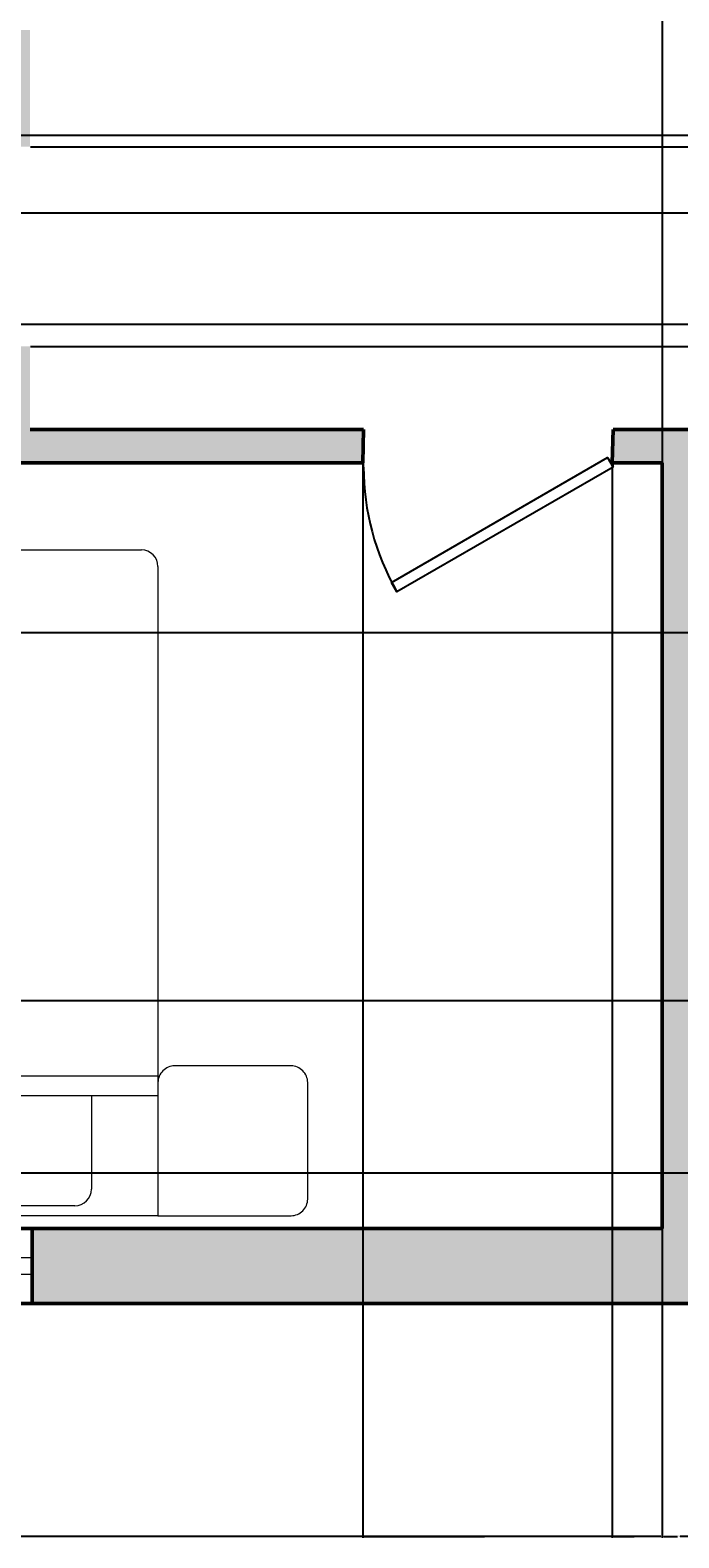
# Model space of a CAD drawing. Units: inches. Extents: x 1869 to 2483, y 2084 to 2479.
# Tile 2 of 7: x 2010 to 2088, y 2084 to 2265. Entities that reach past the tile are written whole.
import ezdxf

# ---------------------------------------------------------------- set-up
doc = ezdxf.new("R2010")
doc.units = ezdxf.units.IN
for name, color, linetype, lineweight in [('A-ANNO-DIMS', 2, 'Continuous', 18), ('A-DOOR', 3, 'Continuous', 25), ('A-FURN', 8, 'Continuous', 18), ('A-GLAZ', 4, 'Continuous', 18), ('A-WALL', 7, 'Continuous', 50)]:
    doc.layers.add(name, color=color, linetype=linetype, lineweight=lineweight)
doc.layers.add('A-WALL-PATT', color=18, linetype='Continuous', lineweight=13, true_color=0x000000)
doc.styles.get("Standard").update_dxf_attribs({"font": 'arial.ttf'})
doc.dimstyles.get("Standard").update_dxf_attribs({"dimtxt": 0.18, "dimasz": 0.18, "dimexe": 0.18, "dimexo": 0.0625, "dimgap": 0.09, "dimtad": 0, "dimtih": 1, "dimtoh": 1, "dimdec": 4, "dimzin": 0, "dimdsep": 46, "dimtxsty": 'Standard', "dimcen": 0.09, "dimadec": 0, "dimazin": 0, "dimtfac": 1, "dimtdec": 4, "dimtofl": 0, "dimtmove": 0, "dimatfit": 3, "dimfxl": 1, "dimtolj": 1, "dimtzin": 0, "dimarcsym": 0})

# ---------------------------------------------------------------- blocks, each defined once
blk = doc.blocks.new('Bed - Queen')
for p, q in [((0, -78), (0, 0)), ((0, 0), (60, 0)), ((60, 0), (60, -78)), ((10, -1.2), (26.8, -1.2)), ((33.2, -1.2), (50, -1.2)), ((8, -14.4), (8, -3.2)), ((28.8, -3.2), (28.8, -14.4)), ((31.2, -14.4), (31.2, -3.2)), ((52, -3.2), (52, -14.4)), ((0, -14.4), (44.8, -14.4)), ((60, -29.6), (44.8, -14.4)), ((44.8, -14.4), (44.8, -27.6)), ((44.8, -16.8), (0, -16.8)), ((50, -16.4), (46.8, -16.4)), ((46.8, -29.6), (60, -29.6)), ((58, -80), (2, -80))]:
    blk.add_line(p, q)
for points in [[(0, 0), (-16, 0, 0.414214), (-18, -2), (-18, -16, 0.414214), (-16, -18), (-2, -18, 0.414214), (0, -16)], [(75.96, 0.02), (59.96, 0.02), (59.96, -15.98, 0.414214), (61.96, -17.98), (75.96, -17.98, 0.414214), (77.96, -15.98), (77.96, -1.98, 0.414214)]]:
    blk.add_lwpolyline(points, format="xyb", close=True)
for centre, start, end in [((10, -3.2), 90, 180), ((26.8, -3.2), 0, 90), ((33.2, -3.2), 90, 180), ((50, -3.2), 0, 90), ((50, -14.4), 270, 0), ((46.8, -27.6), 180, 270), ((2, -78), 180, 270), ((58, -78), 270, 0)]:
    blk.add_arc(centre, 2, start, end)
blk = doc.blocks.new('*U14')
for p, q in [((-40, 0), (-40, 6)), ((0, 0), (0, 6))]:
    blk.add_line(p, q)
blk.add_lwpolyline([(0, 0), (-34.64, -20), (-35.52, -18.48), (-0.88, 1.52)], close=True)
blk.add_arc((0, 0), 40, 180, 210)
blk = doc.blocks.new('WIN-GLAZING-48IN')
for p, q in [((0, 2), (48, 2)), ((0, 0), (48, 0))]:
    blk.add_line(p, q)
blk = doc.blocks.new('*D40')
at = {"layer": 'A-ANNO-DIMS', "color": 0, "lineweight": -2, "transparency": 16777216}
for p, q in [((1906.08, 2120.66), (1906.08, 2083.54)), ((2086.08, 2120.66), (2086.08, 2083.54)), ((1906.26, 2083.72), (1995.8, 2083.72)), ((2085.9, 2083.72), (1996.36, 2083.72))]:
    blk.add_line(p, q, dxfattribs=at)
at = {"layer": 'A-ANNO-DIMS', "color": 0, "transparency": 16777216}
for points in [[(1906.26, 2083.75), (1906.26, 2083.69), (1906.08, 2083.72)], [(2085.9, 2083.75), (2085.9, 2083.69), (2086.08, 2083.72)]]:
    blk.add_solid(points, dxfattribs=at)
at = {"layer": 'Defpoints', "color": 0, "transparency": 16777216}
for p in [(1906.08, 2120.72), (2086.08, 2120.72), (2086.08, 2083.72)]:
    blk.add_point(p, dxfattribs=at)
at = {"layer": 'A-ANNO-DIMS', "color": 0, "transparency": 16777216, "insert": (1996.08, 2083.72), "char_height": 0.18, "attachment_point": 5}
blk.add_mtext('\\A1;180', dxfattribs=at)
blk = doc.blocks.new('*D57')
at = {"layer": 'A-ANNO-DIMS', "color": 0, "lineweight": -2, "transparency": 16777216}
for p, q in [((2446.02, 2296.72), (1868.9, 2296.72)), ((1869.08, 2296.54), (1869.08, 2274.58)), ((1869.08, 2252.25), (1869.08, 2274.22)), ((2446.02, 2252.07), (1868.9, 2252.07))]:
    blk.add_line(p, q, dxfattribs=at)
at = {"layer": 'A-ANNO-DIMS', "color": 0, "transparency": 16777216}
for points in [[(1869.05, 2296.54), (1869.11, 2296.54), (1869.08, 2296.72)], [(1869.05, 2252.25), (1869.11, 2252.25), (1869.08, 2252.07)]]:
    blk.add_solid(points, dxfattribs=at)
at = {"layer": 'Defpoints', "color": 0, "transparency": 16777216}
for p in [(1869.08, 2296.72), (2446.08, 2296.72), (2446.08, 2252.07)]:
    blk.add_point(p, dxfattribs=at)
at = {"layer": 'A-ANNO-DIMS', "color": 0, "transparency": 16777216, "insert": (1869.08, 2274.4), "char_height": 0.18, "attachment_point": 5}
blk.add_mtext('\\A1;44.65', dxfattribs=at)
blk = doc.blocks.new('*D63')
at = {"layer": 'A-ANNO-DIMS', "color": 0, "lineweight": -2, "transparency": 16777216}
for p, q in [((2348.34, 2272.72), (1868.9, 2272.72)), ((1869.08, 2272.54), (1869.08, 2257.91)), ((1869.08, 2242.9), (1869.08, 2257.54)), ((2348.34, 2242.72), (1868.9, 2242.72))]:
    blk.add_line(p, q, dxfattribs=at)
at = {"layer": 'A-ANNO-DIMS', "color": 0, "transparency": 16777216}
for points in [[(1869.05, 2272.54), (1869.11, 2272.54), (1869.08, 2272.72)], [(1869.05, 2242.9), (1869.11, 2242.9), (1869.08, 2242.72)]]:
    blk.add_solid(points, dxfattribs=at)
at = {"layer": 'Defpoints', "color": 0, "transparency": 16777216}
for p in [(1869.08, 2272.72), (2348.4, 2272.72), (2348.4, 2242.72)]:
    blk.add_point(p, dxfattribs=at)
at = {"layer": 'A-ANNO-DIMS', "color": 0, "transparency": 16777216, "insert": (1869.08, 2257.72), "char_height": 0.18, "attachment_point": 5}
blk.add_mtext('\\A1;30', dxfattribs=at)
blk = doc.blocks.new('*D66')
at = {"layer": 'A-ANNO-DIMS', "color": 0, "lineweight": -2, "transparency": 16777216}
for p, q in [((2050.07, 2212.66), (2050.07, 2083.54)), ((2080.08, 2212.66), (2080.08, 2083.54)), ((2050.25, 2083.72), (2064.7, 2083.72)), ((2079.9, 2083.72), (2065.45, 2083.72))]:
    blk.add_line(p, q, dxfattribs=at)
at = {"layer": 'A-ANNO-DIMS', "color": 0, "transparency": 16777216}
for points in [[(2050.25, 2083.75), (2050.25, 2083.69), (2050.07, 2083.72)], [(2079.9, 2083.75), (2079.9, 2083.69), (2080.08, 2083.72)]]:
    blk.add_solid(points, dxfattribs=at)
at = {"layer": 'Defpoints', "color": 0, "transparency": 16777216}
for p in [(2050.07, 2212.72), (2080.08, 2212.72), (2080.08, 2083.72)]:
    blk.add_point(p, dxfattribs=at)
at = {"layer": 'A-ANNO-DIMS', "color": 0, "transparency": 16777216, "insert": (2065.07, 2083.72), "char_height": 0.18, "attachment_point": 5}
blk.add_mtext('\\A1;30.01', dxfattribs=at)
blk = doc.blocks.new('*D68')
at = {"layer": 'A-ANNO-DIMS', "color": 0, "lineweight": -2, "transparency": 16777216}
for p, q in [((2010.14, 2250.72), (2483.26, 2250.72)), ((2483.08, 2250.54), (2483.08, 2238.9)), ((2483.08, 2226.9), (2483.08, 2238.54)), ((2010.14, 2226.72), (2483.26, 2226.72))]:
    blk.add_line(p, q, dxfattribs=at)
at = {"layer": 'A-ANNO-DIMS', "color": 0, "transparency": 16777216}
for points in [[(2483.05, 2250.54), (2483.11, 2250.54), (2483.08, 2250.72)], [(2483.05, 2226.9), (2483.11, 2226.9), (2483.08, 2226.72)]]:
    blk.add_solid(points, dxfattribs=at)
at = {"layer": 'Defpoints', "color": 0, "transparency": 16777216}
for p in [(2010.08, 2250.72), (2483.08, 2250.72), (2010.08, 2226.72)]:
    blk.add_point(p, dxfattribs=at)
at = {"layer": 'A-ANNO-DIMS', "color": 0, "transparency": 16777216, "insert": (2483.08, 2238.72), "char_height": 0.18, "attachment_point": 5}
blk.add_mtext('\\A1;24', dxfattribs=at)
blk = doc.blocks.new('*D72')
at = {"layer": 'A-ANNO-DIMS', "color": 0, "lineweight": -2, "transparency": 16777216}
for p, q in [((2086.08, 2300.66), (2086.08, 2083.54)), ((2090.08, 2296.66), (2090.08, 2083.54)), ((2086.26, 2083.72), (2087.93, 2083.72)), ((2089.9, 2083.72), (2088.23, 2083.72))]:
    blk.add_line(p, q, dxfattribs=at)
at = {"layer": 'A-ANNO-DIMS', "color": 0, "transparency": 16777216}
for points in [[(2086.26, 2083.75), (2086.26, 2083.69), (2086.08, 2083.72)], [(2089.9, 2083.75), (2089.9, 2083.69), (2090.08, 2083.72)]]:
    blk.add_solid(points, dxfattribs=at)
at = {"layer": 'Defpoints', "color": 0, "transparency": 16777216}
for p in [(2086.08, 2300.72), (2090.08, 2296.72), (2090.08, 2083.72)]:
    blk.add_point(p, dxfattribs=at)
at = {"layer": 'A-ANNO-DIMS', "color": 0, "transparency": 16777216, "insert": (2088.08, 2083.72), "char_height": 0.18, "attachment_point": 5}
blk.add_mtext('\\A1;4', dxfattribs=at)
blk = doc.blocks.new('*D86')
at = {"layer": 'A-ANNO-DIMS', "color": 0, "lineweight": -2, "transparency": 16777216}
for p, q in [((2241.99, 2229.37), (1868.9, 2229.37)), ((1869.08, 2229.19), (1869.08, 2178.55)), ((1869.08, 2127.55), (1869.08, 2178.19)), ((2241.99, 2127.37), (1868.9, 2127.37))]:
    blk.add_line(p, q, dxfattribs=at)
at = {"layer": 'A-ANNO-DIMS', "color": 0, "transparency": 16777216}
for points in [[(1869.05, 2229.19), (1869.11, 2229.19), (1869.08, 2229.37)], [(1869.05, 2127.55), (1869.11, 2127.55), (1869.08, 2127.37)]]:
    blk.add_solid(points, dxfattribs=at)
at = {"layer": 'Defpoints', "color": 0, "transparency": 16777216}
for p in [(2242.05, 2229.37), (1869.08, 2127.37), (2242.05, 2127.37)]:
    blk.add_point(p, dxfattribs=at)
at = {"layer": 'A-ANNO-DIMS', "color": 0, "transparency": 16777216, "insert": (1869.08, 2178.37), "char_height": 0.18, "attachment_point": 5}
blk.add_mtext('\\A1;102', dxfattribs=at)
blk = doc.blocks.new('*D89')
at = {"layer": 'A-ANNO-DIMS', "color": 0, "lineweight": -2, "transparency": 16777216}
for p, q in [((2080.08, 2212.66), (2080.08, 2083.54)), ((2086.08, 2212.66), (2086.08, 2083.54)), ((2080.26, 2083.72), (2082.69, 2083.72)), ((2085.9, 2083.72), (2083.47, 2083.72))]:
    blk.add_line(p, q, dxfattribs=at)
at = {"layer": 'A-ANNO-DIMS', "color": 0, "transparency": 16777216}
for points in [[(2080.26, 2083.75), (2080.26, 2083.69), (2080.08, 2083.72)], [(2085.9, 2083.75), (2085.9, 2083.69), (2086.08, 2083.72)]]:
    blk.add_solid(points, dxfattribs=at)
at = {"layer": 'Defpoints', "color": 0, "transparency": 16777216}
for p in [(2080.08, 2212.72), (2086.08, 2212.72), (2086.08, 2083.72)]:
    blk.add_point(p, dxfattribs=at)
at = {"layer": 'A-ANNO-DIMS', "color": 0, "transparency": 16777216, "insert": (2083.08, 2083.72), "char_height": 0.18, "attachment_point": 5}
blk.add_mtext('\\A1;6.002', dxfattribs=at)
blk = doc.blocks.new('*D90')
at = {"layer": 'A-ANNO-DIMS', "color": 0, "lineweight": -2, "transparency": 16777216}
for p, q in [((2190.22, 2192.3), (1868.9, 2192.3)), ((1869.08, 2192.12), (1869.08, 2170.36)), ((1869.08, 2148.24), (1869.08, 2170)), ((2190.22, 2148.06), (1868.9, 2148.06))]:
    blk.add_line(p, q, dxfattribs=at)
at = {"layer": 'A-ANNO-DIMS', "color": 0, "transparency": 16777216}
for points in [[(1869.05, 2192.12), (1869.11, 2192.12), (1869.08, 2192.3)], [(1869.05, 2148.24), (1869.11, 2148.24), (1869.08, 2148.06)]]:
    blk.add_solid(points, dxfattribs=at)
at = {"layer": 'Defpoints', "color": 0, "transparency": 16777216}
for p in [(1869.08, 2192.3), (2190.29, 2192.3), (2190.29, 2148.06)]:
    blk.add_point(p, dxfattribs=at)
at = {"layer": 'A-ANNO-DIMS', "color": 0, "transparency": 16777216, "insert": (1869.08, 2170.18), "char_height": 0.18, "attachment_point": 5}
blk.add_mtext('\\A1;44.24', dxfattribs=at)

msp = doc.modelspace()

# ---------------------------------------------------------------- hatches: boundary and pattern name
at = {"layer": 'A-WALL-PATT'}
h = msp.add_hatch(color=256, dxfattribs=at)
h.dxf.hatch_style = 1
h.paths.add_polyline_path([(1998.5221, 2429.7235), (1897.0799, 2429.7235), (1897.0799, 2252.2488), (1906.0799, 2252.2488), (1906.0799, 2260.7235), (1966.0799, 2260.7235), (1966.0799, 2216.7235), (1960.0791, 2216.7235), (1960.0161, 2212.7235), (2050.0707, 2212.7235), (2050.1612, 2216.7235), (2010.0799, 2216.7235), (2010.0799, 2226.7235), (2006.0799, 2226.7235), (2006.0799, 2216.7235), (1970.0799, 2216.7235), (1970.0799, 2260.7235), (2006.0799, 2260.7235), (2006.0799, 2250.7235), (2010.0799, 2250.7235), (2010.0799, 2264.7235), (1906.0799, 2264.7235), (1906.0799, 2336.7235), (1920.0799, 2336.7235), (1920.0799, 2340.7235), (1906.0799, 2340.7235), (1906.0799, 2420.7235), (1950.0799, 2420.7235), (1950.0799, 2340.7235), (1944.0799, 2340.7235), (1944.0799, 2336.7235), (1950.0799, 2336.7235), (1950.0799, 2296.7235), (2050.0799, 2296.7235), (2050.0799, 2300.7235), (1954.0799, 2300.7235), (1954.0799, 2420.7235), (1998.5221, 2420.7235)])
h = msp.add_hatch(color=256, dxfattribs=at)
h.dxf.hatch_style = 1
h.paths.add_polyline_path([(2152.0799, 2118.9235), (2152.0799, 2120.7235), (2090.0799, 2120.7235), (2090.0799, 2216.7235), (2080.1689, 2216.7235), (2080.1689, 2212.7235), (2086.0799, 2212.7235), (2086.0799, 2120.7235), (2010.3331, 2120.7235), (2010.3331, 2111.7235), (2152.0799, 2111.7235)])

# ---------------------------------------------------------------- linework, layer by layer
at = {"layer": 'A-WALL'}
for p, q in [((2050.1612, 2216.7235), (2010.0799, 2216.7235)), ((2050.0707, 2212.7235), (2050.1612, 2216.7235)), ((2080.0783, 2212.7235), (2080.1689, 2216.7235)), ((2090.0799, 2216.7235), (2080.1689, 2216.7235)), ((2050.0707, 2212.7235), (1960.0161, 2212.7235)), ((2086.0799, 2212.7235), (2080.0783, 2212.7235)), ((2086.0799, 2120.7235), (2086.0799, 2212.7235)), ((2086.0799, 2120.7235), (1906.0799, 2120.7235)), ((2010.3331, 2120.7235), (2010.3331, 2111.7235))]:
    msp.add_line(p, q, dxfattribs=at)
msp.add_lwpolyline([(2152.0799, 2111.7235), (1897.0799, 2111.7235), (1897.0799, 2429.7235), (2455.0799, 2429.7235), (2455.0799, 2111.7235), (2200.0799, 2111.7235)], dxfattribs=at)

# ---------------------------------------------------------------- block references
at = {"layer": 'A-DOOR', "xscale": 0.75, "yscale": 0.75, "zscale": 0.75}
msp.add_blockref('*U14', (2080.1689, 2212.2235), dxfattribs=at)
at = {"layer": 'A-FURN', "rotation": 180}
msp.add_blockref('Bed - Queen', (2025.4526, 2122.2569), dxfattribs=at)
at = {"layer": 'A-GLAZ'}
msp.add_blockref('WIN-GLAZING-48IN', (1962.333, 2115.224), dxfattribs=at)

# ---------------------------------------------------------------- dimensions: what is measured, and where the dimension line sits
at = {"layer": 'A-ANNO-DIMS'}
for base, p1, p2, override, picture, middle in [((2090.0799, 2083.7235), (2086.0799, 2300.7235), (2090.0799, 2296.7235), {"dimdec": 0, "dimlfac": 1, "dimrnd": 0, "dimzin": 0, "dimdsep": 46, "dimlunit": 2}, '*D72', (2088.0799, 2083.7235)), ((2080.0783, 2083.7235), (2050.0707, 2212.7235), (2080.0783, 2212.7235), {"dimdec": 2, "dimlfac": 1, "dimrnd": 0, "dimzin": 0, "dimdsep": 46, "dimlunit": 2}, '*D66', (2065.0745, 2083.7235)), ((2086.0799, 2083.7235), (2080.0783, 2212.7235), (2086.0799, 2212.7235), {"dimdec": 3, "dimlfac": 1, "dimrnd": 0, "dimzin": 0, "dimdsep": 46, "dimlunit": 2}, '*D89', (2083.0791, 2083.7235)), ((2086.0799, 2083.7235), (1906.0799, 2120.7235), (2086.0799, 2120.7235), {"dimdec": 0, "dimlfac": 1, "dimrnd": 0, "dimzin": 0, "dimdsep": 46, "dimlunit": 2}, '*D40', (1996.0799, 2083.7235))]:
    dim = msp.add_linear_dim(base=base, p1=p1, p2=p2, dimstyle='Standard', override=override, dxfattribs=at)
    dim.commit()
    dim.dimension.update_dxf_attribs({"geometry": picture, "text_midpoint": middle})
for base, p1, p2, override, picture, middle in [((1869.0799, 2296.7235), (2446.0799, 2252.0706), (2446.0799, 2296.7235), {"dimdec": 2, "dimlfac": 1, "dimrnd": 0, "dimzin": 0, "dimdsep": 46, "dimlunit": 2}, '*D57', (1869.0799, 2274.3971)), ((1869.0799, 2272.7235), (2348.3982, 2242.7235), (2348.3982, 2272.7235), {"dimdec": 0, "dimlfac": 1, "dimrnd": 0, "dimzin": 0, "dimdsep": 46, "dimlunit": 2}, '*D63', (1869.0799, 2257.7235)), ((2483.0799, 2250.7235), (2010.0799, 2226.7235), (2010.0799, 2250.7235), {"dimdec": 0, "dimlfac": 1, "dimrnd": 0, "dimzin": 0, "dimdsep": 46, "dimlunit": 2}, '*D68', (2483.0799, 2238.7235)), ((1869.0799, 2127.3727), (2242.0537, 2229.3727), (2242.0537, 2127.3727), {"dimdec": 0, "dimlfac": 1, "dimrnd": 0, "dimzin": 0, "dimdsep": 46, "dimlunit": 2}, '*D86', (1869.0799, 2178.3727)), ((1869.0799, 2192.3029), (2190.2869, 2148.0595), (2190.2869, 2192.3029), {"dimdec": 2, "dimlfac": 1, "dimrnd": 0, "dimzin": 0, "dimdsep": 46, "dimlunit": 2}, '*D90', (1869.0799, 2170.1812))]:
    dim = msp.add_linear_dim(base=base, p1=p1, p2=p2, angle=90, dimstyle='Standard', override=override, dxfattribs=at)
    dim.commit()
    dim.dimension.update_dxf_attribs({"geometry": picture, "text_midpoint": middle})

doc.saveas('drawing.dxf')
